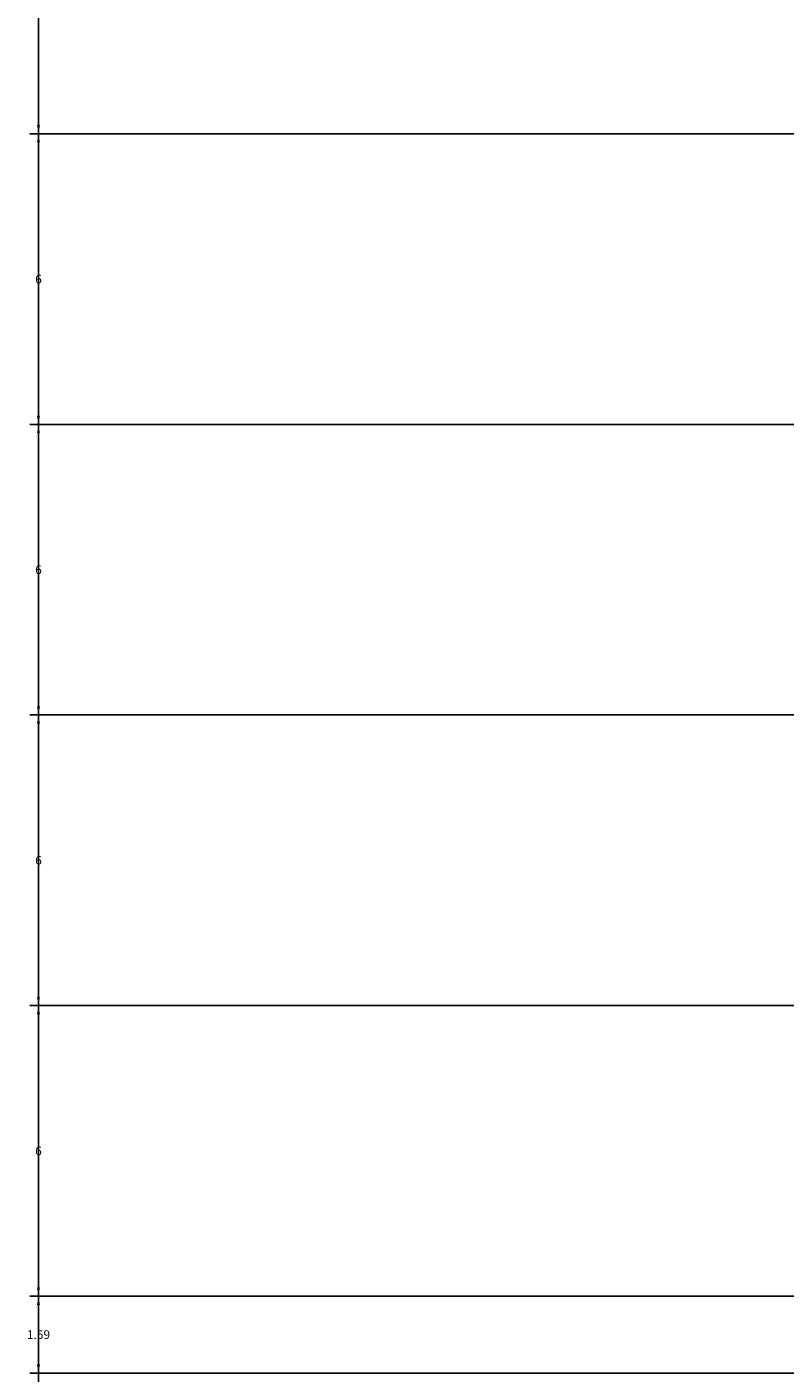
# Model space of a CAD drawing. Units: feet. Extents: x 2695 to 2912, y 795 to 1139.
# Tile 35 of 83: x 2695 to 2710, y 937 to 965. Entities that reach past the tile are written whole.
import ezdxf

# ---------------------------------------------------------------- set-up
doc = ezdxf.new("R2010")
doc.units = ezdxf.units.FT
doc.layers.add('A-ANNO-DIMS', color=2, linetype='Continuous', lineweight=18)
doc.styles.get("Standard").update_dxf_attribs({"font": 'arial.ttf'})
doc.dimstyles.get("Standard").update_dxf_attribs({"dimtxt": 0.18, "dimasz": 0.18, "dimexe": 0.18, "dimexo": 0.0625, "dimgap": 0.09, "dimtad": 0, "dimtih": 1, "dimtoh": 1, "dimdec": 1, "dimzin": 0, "dimdsep": 46, "dimlunit": 3, "dimtxsty": 'Standard', "dimcen": 0.09, "dimadec": 0, "dimazin": 0, "dimtfac": 1, "dimtdec": 1, "dimtofl": 0, "dimtmove": 0, "dimatfit": 3, "dimfxl": 1, "dimtolj": 1, "dimtzin": 0, "dimarcsym": 0})

# ---------------------------------------------------------------- blocks, each defined once
blk = doc.blocks.new('*D12')
at = {"layer": 'A-ANNO-DIMS', "color": 0, "lineweight": -2, "transparency": 16777216}
for p, q in [((2710.574, 1122.931), (2694.681, 1122.931)), ((2694.861, 1122.751), (2694.861, 967.113)), ((2694.861, 811.111), (2694.861, 966.749)), ((2710.574, 810.931), (2694.681, 810.931))]:
    blk.add_line(p, q, dxfattribs=at)
at = {"layer": 'A-ANNO-DIMS', "color": 0, "transparency": 16777216}
for points in [[(2694.831, 1122.751), (2694.891, 1122.751), (2694.861, 1122.931)], [(2694.831, 811.111), (2694.891, 811.111), (2694.861, 810.931)]]:
    blk.add_solid(points, dxfattribs=at)
at = {"layer": 'Defpoints', "color": 0, "transparency": 16777216}
for p in [(2694.861, 1122.931), (2710.636, 1122.931), (2710.636, 810.931)]:
    blk.add_point(p, dxfattribs=at)
at = {"layer": 'A-ANNO-DIMS', "color": 0, "transparency": 16777216, "insert": (2694.861, 966.931), "char_height": 0.18, "attachment_point": 5}
blk.add_mtext('\\A1;312', dxfattribs=at)
blk = doc.blocks.new('*D27')
at = {"layer": 'A-ANNO-DIMS', "color": 0, "lineweight": -2, "transparency": 16777216}
for p, q in [((2730.646, 938.518), (2694.681, 938.518)), ((2694.861, 938.338), (2694.861, 937.906)), ((2694.861, 937.111), (2694.861, 937.542)), ((2730.646, 936.931), (2694.681, 936.931))]:
    blk.add_line(p, q, dxfattribs=at)
at = {"layer": 'A-ANNO-DIMS', "color": 0, "transparency": 16777216}
for points in [[(2694.831, 938.338), (2694.891, 938.338), (2694.861, 938.518)], [(2694.831, 937.111), (2694.891, 937.111), (2694.861, 936.931)]]:
    blk.add_solid(points, dxfattribs=at)
at = {"layer": 'Defpoints', "color": 0, "transparency": 16777216}
for p in [(2694.861, 938.518), (2730.708, 938.518), (2730.708, 936.931)]:
    blk.add_point(p, dxfattribs=at)
at = {"layer": 'A-ANNO-DIMS', "color": 0, "transparency": 16777216, "insert": (2694.861, 937.724), "char_height": 0.18, "attachment_point": 5}
blk.add_mtext('\\A1;1.59', dxfattribs=at)
blk = doc.blocks.new('*D28')
at = {"layer": 'A-ANNO-DIMS', "color": 0, "lineweight": -2, "transparency": 16777216}
for p, q in [((2730.646, 944.518), (2694.681, 944.518)), ((2694.861, 944.338), (2694.861, 941.7)), ((2694.861, 938.698), (2694.861, 941.336)), ((2730.646, 938.518), (2694.681, 938.518))]:
    blk.add_line(p, q, dxfattribs=at)
at = {"layer": 'A-ANNO-DIMS', "color": 0, "transparency": 16777216}
for points in [[(2694.831, 944.338), (2694.891, 944.338), (2694.861, 944.518)], [(2694.831, 938.698), (2694.891, 938.698), (2694.861, 938.518)]]:
    blk.add_solid(points, dxfattribs=at)
at = {"layer": 'Defpoints', "color": 0, "transparency": 16777216}
for p in [(2694.861, 944.518), (2730.708, 944.518), (2730.708, 938.518)]:
    blk.add_point(p, dxfattribs=at)
at = {"layer": 'A-ANNO-DIMS', "color": 0, "transparency": 16777216, "insert": (2694.861, 941.518), "char_height": 0.18, "attachment_point": 5}
blk.add_mtext('\\A1;6', dxfattribs=at)
blk = doc.blocks.new('*D29')
at = {"layer": 'A-ANNO-DIMS', "color": 0, "lineweight": -2, "transparency": 16777216}
for p, q in [((2730.646, 950.518), (2694.681, 950.518)), ((2694.861, 950.338), (2694.861, 947.7)), ((2694.861, 944.698), (2694.861, 947.336)), ((2730.646, 944.518), (2694.681, 944.518))]:
    blk.add_line(p, q, dxfattribs=at)
at = {"layer": 'A-ANNO-DIMS', "color": 0, "transparency": 16777216}
for points in [[(2694.831, 950.338), (2694.891, 950.338), (2694.861, 950.518)], [(2694.831, 944.698), (2694.891, 944.698), (2694.861, 944.518)]]:
    blk.add_solid(points, dxfattribs=at)
at = {"layer": 'Defpoints', "color": 0, "transparency": 16777216}
for p in [(2694.861, 950.518), (2730.708, 950.518), (2730.708, 944.518)]:
    blk.add_point(p, dxfattribs=at)
at = {"layer": 'A-ANNO-DIMS', "color": 0, "transparency": 16777216, "insert": (2694.861, 947.518), "char_height": 0.18, "attachment_point": 5}
blk.add_mtext('\\A1;6', dxfattribs=at)
blk = doc.blocks.new('*D30')
at = {"layer": 'A-ANNO-DIMS', "color": 0, "lineweight": -2, "transparency": 16777216}
for p, q in [((2730.646, 956.518), (2694.681, 956.518)), ((2694.861, 956.338), (2694.861, 953.7)), ((2694.861, 950.698), (2694.861, 953.336)), ((2730.646, 950.518), (2694.681, 950.518))]:
    blk.add_line(p, q, dxfattribs=at)
at = {"layer": 'A-ANNO-DIMS', "color": 0, "transparency": 16777216}
for points in [[(2694.831, 956.338), (2694.891, 956.338), (2694.861, 956.518)], [(2694.831, 950.698), (2694.891, 950.698), (2694.861, 950.518)]]:
    blk.add_solid(points, dxfattribs=at)
at = {"layer": 'Defpoints', "color": 0, "transparency": 16777216}
for p in [(2694.861, 956.518), (2730.708, 956.518), (2730.708, 950.518)]:
    blk.add_point(p, dxfattribs=at)
at = {"layer": 'A-ANNO-DIMS', "color": 0, "transparency": 16777216, "insert": (2694.861, 953.518), "char_height": 0.18, "attachment_point": 5}
blk.add_mtext('\\A1;6', dxfattribs=at)
blk = doc.blocks.new('*D31')
at = {"layer": 'A-ANNO-DIMS', "color": 0, "lineweight": -2, "transparency": 16777216}
for p, q in [((2730.646, 962.518), (2694.681, 962.518)), ((2694.861, 962.338), (2694.861, 959.7)), ((2694.861, 956.698), (2694.861, 959.336)), ((2730.646, 956.518), (2694.681, 956.518))]:
    blk.add_line(p, q, dxfattribs=at)
at = {"layer": 'A-ANNO-DIMS', "color": 0, "transparency": 16777216}
for points in [[(2694.831, 962.338), (2694.891, 962.338), (2694.861, 962.518)], [(2694.831, 956.698), (2694.891, 956.698), (2694.861, 956.518)]]:
    blk.add_solid(points, dxfattribs=at)
at = {"layer": 'Defpoints', "color": 0, "transparency": 16777216}
for p in [(2694.861, 962.518), (2730.708, 962.518), (2730.708, 956.518)]:
    blk.add_point(p, dxfattribs=at)
at = {"layer": 'A-ANNO-DIMS', "color": 0, "transparency": 16777216, "insert": (2694.861, 959.518), "char_height": 0.18, "attachment_point": 5}
blk.add_mtext('\\A1;6', dxfattribs=at)
blk = doc.blocks.new('*D32')
at = {"layer": 'A-ANNO-DIMS', "color": 0, "lineweight": -2, "transparency": 16777216}
for p, q in [((2730.646, 968.518), (2694.681, 968.518)), ((2694.861, 968.338), (2694.861, 965.7)), ((2694.861, 962.698), (2694.861, 965.336)), ((2730.646, 962.518), (2694.681, 962.518))]:
    blk.add_line(p, q, dxfattribs=at)
at = {"layer": 'A-ANNO-DIMS', "color": 0, "transparency": 16777216}
for points in [[(2694.831, 968.338), (2694.891, 968.338), (2694.861, 968.518)], [(2694.831, 962.698), (2694.891, 962.698), (2694.861, 962.518)]]:
    blk.add_solid(points, dxfattribs=at)
at = {"layer": 'Defpoints', "color": 0, "transparency": 16777216}
for p in [(2694.861, 968.518), (2730.708, 968.518), (2730.708, 962.518)]:
    blk.add_point(p, dxfattribs=at)
at = {"layer": 'A-ANNO-DIMS', "color": 0, "transparency": 16777216, "insert": (2694.861, 965.518), "char_height": 0.18, "attachment_point": 5}
blk.add_mtext('\\A1;6', dxfattribs=at)

msp = doc.modelspace()

# ---------------------------------------------------------------- dimensions: what is measured, and where the dimension line sits
at = {"layer": 'A-ANNO-DIMS'}
for base, p1, p2, override, picture, middle in [((2694.8611, 1122.9306), (2710.6361, 810.9306), (2710.6361, 1122.9306), {"dimdec": 0, "dimlfac": 1, "dimrnd": 0, "dimzin": 0, "dimdsep": 46, "dimlunit": 2}, '*D12', (2694.8611, 966.9306)), ((2694.8611, 968.5179), (2730.7081, 962.5179), (2730.7081, 968.5179), {"dimdec": 0, "dimlfac": 1, "dimrnd": 0, "dimzin": 0, "dimdsep": 46, "dimlunit": 2}, '*D32', (2694.8611, 965.5179)), ((2694.8611, 962.5179), (2730.7081, 956.5179), (2730.7081, 962.5179), {"dimdec": 0, "dimlfac": 1, "dimrnd": 0, "dimzin": 0, "dimdsep": 46, "dimlunit": 2}, '*D31', (2694.8611, 959.5179)), ((2694.8611, 956.5179), (2730.7081, 950.5179), (2730.7081, 956.5179), {"dimdec": 0, "dimlfac": 1, "dimrnd": 0, "dimzin": 0, "dimdsep": 46, "dimlunit": 2}, '*D30', (2694.8611, 953.5179)), ((2694.8611, 950.5179), (2730.7081, 944.5179), (2730.7081, 950.5179), {"dimdec": 0, "dimlfac": 1, "dimrnd": 0, "dimzin": 0, "dimdsep": 46, "dimlunit": 2}, '*D29', (2694.8611, 947.5179)), ((2694.8611, 944.5179), (2730.7081, 938.5179), (2730.7081, 944.5179), {"dimdec": 0, "dimlfac": 1, "dimrnd": 0, "dimzin": 0, "dimdsep": 46, "dimlunit": 2}, '*D28', (2694.8611, 941.5179)), ((2694.8611, 938.5179), (2730.7081, 936.9306), (2730.7081, 938.5179), {"dimdec": 2, "dimlfac": 1, "dimrnd": 0, "dimzin": 0, "dimdsep": 46, "dimlunit": 2}, '*D27', (2694.8611, 937.7242))]:
    dim = msp.add_linear_dim(base=base, p1=p1, p2=p2, angle=90, dimstyle='Standard', override=override, dxfattribs=at)
    dim.commit()
    dim.dimension.update_dxf_attribs({"geometry": picture, "text_midpoint": middle})

doc.saveas('drawing.dxf')
